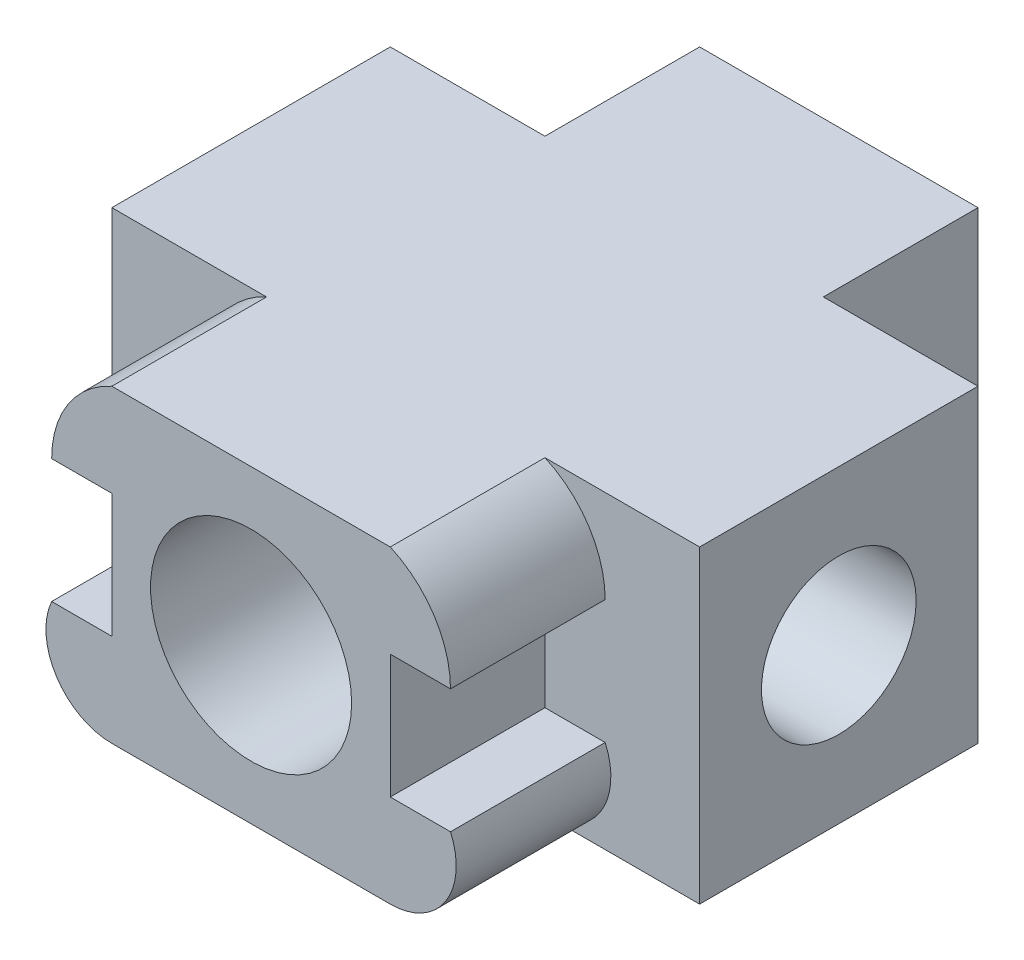
ISO-10303-21;
HEADER;
FILE_DESCRIPTION(('STEP AP214'),'2;1');
FILE_NAME('part.step','',(''),(''),'','','');
FILE_SCHEMA(('AUTOMOTIVE_DESIGN { 1 0 10303 214 1 1 1 1 }'));
ENDSEC;
DATA;
#1=APPLICATION_CONTEXT('core data for automotive mechanical design processes');
#2=APPLICATION_PROTOCOL_DEFINITION('international standard','automotive_design',2000,#1);
#3=PRODUCT_CONTEXT('',#1,'mechanical');
#4=PRODUCT('Part','Part','',(#3));
#5=PRODUCT_RELATED_PRODUCT_CATEGORY('part','',(#4));
#6=PRODUCT_DEFINITION_FORMATION('','',#4);
#7=PRODUCT_DEFINITION_CONTEXT('part definition',#1,'design');
#8=PRODUCT_DEFINITION('design','',#6,#7);
#9=PRODUCT_DEFINITION_SHAPE('','',#8);
#10=(LENGTH_UNIT() NAMED_UNIT(*) SI_UNIT(.MILLI.,.METRE.));
#11=(NAMED_UNIT(*) PLANE_ANGLE_UNIT() SI_UNIT($,.RADIAN.));
#12=(NAMED_UNIT(*) SI_UNIT($,.STERADIAN.) SOLID_ANGLE_UNIT());
#13=UNCERTAINTY_MEASURE_WITH_UNIT(LENGTH_MEASURE(1.E-05),#10,'distance_accuracy_value','');
#14=(GEOMETRIC_REPRESENTATION_CONTEXT(3) GLOBAL_UNCERTAINTY_ASSIGNED_CONTEXT((#13)) GLOBAL_UNIT_ASSIGNED_CONTEXT((#10,
#11,#12)) REPRESENTATION_CONTEXT('',''));
#15=CARTESIAN_POINT('',(0.,0.,0.));
#16=DIRECTION('',(0.,0.,1.));
#17=DIRECTION('',(1.,0.,0.));
#18=AXIS2_PLACEMENT_3D('',#15,#16,#17);
#19=CARTESIAN_POINT('',(20.,40.,36.));
#20=DIRECTION('',(0.,0.,-1.));
#21=DIRECTION('',(-1.,0.,0.));
#22=AXIS2_PLACEMENT_3D('',#19,#20,#21);
#23=PLANE('',#22);
#24=CARTESIAN_POINT('',(20.,8.52694245865046,36.));
#25=DIRECTION('',(0.,0.,1.));
#26=DIRECTION('',(1.,0.,0.));
#27=AXIS2_PLACEMENT_3D('',#24,#25,#26);
#28=CIRCLE('',#27,8.52694245865046);
#29=CARTESIAN_POINT('',(20.,0.,36.));
#30=VERTEX_POINT('',#29);
#31=CARTESIAN_POINT('',(12.2124060835447,12.,36.));
#32=VERTEX_POINT('',#31);
#33=EDGE_CURVE('E57',#30,#32,#28,.F.);
#34=ORIENTED_EDGE('',*,*,#33,.T.);
#35=DIRECTION('',(-1.,0.,0.));
#36=VECTOR('',#35,1.);
#37=CARTESIAN_POINT('',(0.,12.,36.));
#38=LINE('',#37,#36);
#39=CARTESIAN_POINT('',(20.,12.,36.));
#40=VERTEX_POINT('',#39);
#41=EDGE_CURVE('E64',#40,#32,#38,.T.);
#42=ORIENTED_EDGE('',*,*,#41,.F.);
#43=DIRECTION('',(0.,-1.,0.));
#44=VECTOR('',#43,1.);
#45=CARTESIAN_POINT('',(20.,40.,36.));
#46=LINE('',#45,#44);
#47=CARTESIAN_POINT('',(20.,28.,36.));
#48=VERTEX_POINT('',#47);
#49=EDGE_CURVE('E47',#48,#40,#46,.T.);
#50=ORIENTED_EDGE('',*,*,#49,.F.);
#51=DIRECTION('',(-1.,0.,0.));
#52=VECTOR('',#51,1.);
#53=CARTESIAN_POINT('',(0.,28.,36.));
#54=LINE('',#53,#52);
#55=CARTESIAN_POINT('',(12.2124060835447,28.,36.));
#56=VERTEX_POINT('',#55);
#57=EDGE_CURVE('E249',#48,#56,#54,.T.);
#58=ORIENTED_EDGE('',*,*,#57,.T.);
#59=CARTESIAN_POINT('',(25.3516774170943,28.,36.));
#60=DIRECTION('',(0.,0.,1.));
#61=DIRECTION('',(1.,0.,0.));
#62=AXIS2_PLACEMENT_3D('',#59,#60,#61);
#63=CIRCLE('',#62,13.1392713335496);
#64=CARTESIAN_POINT('',(20.,40.,36.));
#65=VERTEX_POINT('',#64);
#66=EDGE_CURVE('E248',#56,#65,#63,.F.);
#67=ORIENTED_EDGE('',*,*,#66,.T.);
#68=DIRECTION('',(1.,0.,0.));
#69=VECTOR('',#68,1.);
#70=CARTESIAN_POINT('',(20.,40.,36.));
#71=LINE('',#70,#69);
#72=CARTESIAN_POINT('',(0.,40.,36.));
#73=VERTEX_POINT('',#72);
#74=EDGE_CURVE('E262',#73,#65,#71,.T.);
#75=ORIENTED_EDGE('',*,*,#74,.F.);
#76=DIRECTION('',(0.,-1.,0.));
#77=VECTOR('',#76,1.);
#78=CARTESIAN_POINT('',(0.,40.,36.));
#79=LINE('',#78,#77);
#80=CARTESIAN_POINT('',(0.,0.,36.));
#81=VERTEX_POINT('',#80);
#82=EDGE_CURVE('E11',#73,#81,#79,.T.);
#83=ORIENTED_EDGE('',*,*,#82,.T.);
#84=DIRECTION('',(1.,0.,0.));
#85=VECTOR('',#84,1.);
#86=CARTESIAN_POINT('',(20.,0.,36.));
#87=LINE('',#86,#85);
#88=EDGE_CURVE('E192',#81,#30,#87,.T.);
#89=ORIENTED_EDGE('',*,*,#88,.T.);
#90=EDGE_LOOP('',(#34,#42,#50,#58,#67,#75,#83,#89));
#91=FACE_BOUND('',#90,.T.);
#92=ADVANCED_FACE('F41',(#91),#23,.F.);
#93=CARTESIAN_POINT('',(56.,40.,36.));
#94=DIRECTION('',(-1.,0.,0.));
#95=DIRECTION('',(0.,0.,1.));
#96=AXIS2_PLACEMENT_3D('',#93,#94,#95);
#97=PLANE('',#96);
#98=DIRECTION('',(0.,0.,1.));
#99=VECTOR('',#98,1.);
#100=CARTESIAN_POINT('',(56.,12.,36.));
#101=LINE('',#100,#99);
#102=CARTESIAN_POINT('',(56.,12.,36.));
#103=VERTEX_POINT('',#102);
#104=CARTESIAN_POINT('',(56.,12.,56.));
#105=VERTEX_POINT('',#104);
#106=EDGE_CURVE('E223',#103,#105,#101,.T.);
#107=ORIENTED_EDGE('',*,*,#106,.F.);
#108=DIRECTION('',(0.,-1.,0.));
#109=VECTOR('',#108,1.);
#110=CARTESIAN_POINT('',(56.,40.,36.));
#111=LINE('',#110,#109);
#112=CARTESIAN_POINT('',(56.,28.,36.));
#113=VERTEX_POINT('',#112);
#114=EDGE_CURVE('E328',#113,#103,#111,.T.);
#115=ORIENTED_EDGE('',*,*,#114,.F.);
#116=DIRECTION('',(0.,0.,1.));
#117=VECTOR('',#116,1.);
#118=CARTESIAN_POINT('',(56.,28.,36.));
#119=LINE('',#118,#117);
#120=CARTESIAN_POINT('',(56.,28.,56.));
#121=VERTEX_POINT('',#120);
#122=EDGE_CURVE('E244',#113,#121,#119,.T.);
#123=ORIENTED_EDGE('',*,*,#122,.T.);
#124=DIRECTION('',(0.,-1.,0.));
#125=VECTOR('',#124,1.);
#126=CARTESIAN_POINT('',(56.,40.,56.));
#127=LINE('',#126,#125);
#128=EDGE_CURVE('E335',#121,#105,#127,.T.);
#129=ORIENTED_EDGE('',*,*,#128,.T.);
#130=EDGE_LOOP('',(#107,#115,#123,#129));
#131=FACE_BOUND('',#130,.T.);
#132=ADVANCED_FACE('F404',(#131),#97,.F.);
#133=CARTESIAN_POINT('',(76.,40.,36.));
#134=DIRECTION('',(0.,0.,-1.));
#135=DIRECTION('',(-1.,0.,0.));
#136=AXIS2_PLACEMENT_3D('',#133,#134,#135);
#137=PLANE('',#136);
#138=DIRECTION('',(1.,0.,0.));
#139=VECTOR('',#138,1.);
#140=CARTESIAN_POINT('',(0.,12.,36.));
#141=LINE('',#140,#139);
#142=CARTESIAN_POINT('',(63.7875939164553,12.,36.));
#143=VERTEX_POINT('',#142);
#144=EDGE_CURVE('E217',#103,#143,#141,.T.);
#145=ORIENTED_EDGE('',*,*,#144,.T.);
#146=CARTESIAN_POINT('',(56.,8.52694245865045,36.));
#147=DIRECTION('',(0.,0.,1.));
#148=DIRECTION('',(1.,0.,0.));
#149=AXIS2_PLACEMENT_3D('',#146,#147,#148);
#150=CIRCLE('',#149,8.52694245865045);
#151=CARTESIAN_POINT('',(56.,0.,36.));
#152=VERTEX_POINT('',#151);
#153=EDGE_CURVE('E214',#152,#143,#150,.T.);
#154=ORIENTED_EDGE('',*,*,#153,.F.);
#155=DIRECTION('',(1.,0.,0.));
#156=VECTOR('',#155,1.);
#157=CARTESIAN_POINT('',(76.,0.,36.));
#158=LINE('',#157,#156);
#159=CARTESIAN_POINT('',(76.,0.,36.));
#160=VERTEX_POINT('',#159);
#161=EDGE_CURVE('E299',#152,#160,#158,.T.);
#162=ORIENTED_EDGE('',*,*,#161,.T.);
#163=DIRECTION('',(0.,-1.,0.));
#164=VECTOR('',#163,1.);
#165=CARTESIAN_POINT('',(76.,40.,36.));
#166=LINE('',#165,#164);
#167=CARTESIAN_POINT('',(76.,40.,36.));
#168=VERTEX_POINT('',#167);
#169=EDGE_CURVE('E326',#168,#160,#166,.T.);
#170=ORIENTED_EDGE('',*,*,#169,.F.);
#171=DIRECTION('',(1.,0.,0.));
#172=VECTOR('',#171,1.);
#173=CARTESIAN_POINT('',(76.,40.,36.));
#174=LINE('',#173,#172);
#175=CARTESIAN_POINT('',(56.,40.,36.));
#176=VERTEX_POINT('',#175);
#177=EDGE_CURVE('E280',#176,#168,#174,.T.);
#178=ORIENTED_EDGE('',*,*,#177,.F.);
#179=CARTESIAN_POINT('',(50.6483225829057,28.,36.));
#180=DIRECTION('',(0.,0.,1.));
#181=DIRECTION('',(1.,0.,0.));
#182=AXIS2_PLACEMENT_3D('',#179,#180,#181);
#183=CIRCLE('',#182,13.1392713335496);
#184=CARTESIAN_POINT('',(63.7875939164553,28.,36.));
#185=VERTEX_POINT('',#184);
#186=EDGE_CURVE('E231',#185,#176,#183,.T.);
#187=ORIENTED_EDGE('',*,*,#186,.F.);
#188=DIRECTION('',(1.,0.,0.));
#189=VECTOR('',#188,1.);
#190=CARTESIAN_POINT('',(0.,28.,36.));
#191=LINE('',#190,#189);
#192=EDGE_CURVE('E227',#113,#185,#191,.T.);
#193=ORIENTED_EDGE('',*,*,#192,.F.);
#194=ORIENTED_EDGE('',*,*,#114,.T.);
#195=EDGE_LOOP('',(#145,#154,#162,#170,#178,#187,#193,#194));
#196=FACE_BOUND('',#195,.T.);
#197=ADVANCED_FACE('F391',(#196),#137,.F.);
#198=CARTESIAN_POINT('',(20.,40.,56.));
#199=DIRECTION('',(1.,0.,0.));
#200=DIRECTION('',(0.,0.,-1.));
#201=AXIS2_PLACEMENT_3D('',#198,#199,#200);
#202=PLANE('',#201);
#203=ORIENTED_EDGE('',*,*,#49,.T.);
#204=DIRECTION('',(0.,0.,1.));
#205=VECTOR('',#204,1.);
#206=CARTESIAN_POINT('',(20.,12.,36.));
#207=LINE('',#206,#205);
#208=CARTESIAN_POINT('',(20.,12.,56.));
#209=VERTEX_POINT('',#208);
#210=EDGE_CURVE('E213',#40,#209,#207,.T.);
#211=ORIENTED_EDGE('',*,*,#210,.T.);
#212=DIRECTION('',(0.,-1.,0.));
#213=VECTOR('',#212,1.);
#214=CARTESIAN_POINT('',(20.,40.,56.));
#215=LINE('',#214,#213);
#216=CARTESIAN_POINT('',(20.,28.,56.));
#217=VERTEX_POINT('',#216);
#218=EDGE_CURVE('E331',#217,#209,#215,.T.);
#219=ORIENTED_EDGE('',*,*,#218,.F.);
#220=DIRECTION('',(0.,0.,1.));
#221=VECTOR('',#220,1.);
#222=CARTESIAN_POINT('',(20.,28.,36.));
#223=LINE('',#222,#221);
#224=EDGE_CURVE('E258',#48,#217,#223,.T.);
#225=ORIENTED_EDGE('',*,*,#224,.F.);
#226=EDGE_LOOP('',(#203,#211,#219,#225));
#227=FACE_BOUND('',#226,.T.);
#228=ADVANCED_FACE('F340',(#227),#202,.F.);
#229=CARTESIAN_POINT('',(0.,40.,36.));
#230=DIRECTION('',(1.,0.,0.));
#231=DIRECTION('',(0.,0.,-1.));
#232=AXIS2_PLACEMENT_3D('',#229,#230,#231);
#233=PLANE('',#232);
#234=CARTESIAN_POINT('',(0.,20.,18.));
#235=DIRECTION('',(1.,0.,0.));
#236=DIRECTION('',(0.,0.,-1.));
#237=AXIS2_PLACEMENT_3D('',#234,#235,#236);
#238=CIRCLE('',#237,10.);
#239=CARTESIAN_POINT('',(0.,20.,8.00000000000002));
#240=VERTEX_POINT('',#239);
#241=EDGE_CURVE('E344',#240,#240,#238,.T.);
#242=ORIENTED_EDGE('',*,*,#241,.T.);
#243=EDGE_LOOP('',(#242));
#244=FACE_BOUND('',#243,.T.);
#245=DIRECTION('',(0.,0.,1.));
#246=VECTOR('',#245,1.);
#247=CARTESIAN_POINT('',(0.,0.,36.));
#248=LINE('',#247,#246);
#249=CARTESIAN_POINT('',(0.,0.,0.));
#250=VERTEX_POINT('',#249);
#251=EDGE_CURVE('E256',#250,#81,#248,.T.);
#252=ORIENTED_EDGE('',*,*,#251,.T.);
#253=ORIENTED_EDGE('',*,*,#82,.F.);
#254=DIRECTION('',(0.,0.,1.));
#255=VECTOR('',#254,1.);
#256=CARTESIAN_POINT('',(0.,40.,36.));
#257=LINE('',#256,#255);
#258=CARTESIAN_POINT('',(0.,40.,0.));
#259=VERTEX_POINT('',#258);
#260=EDGE_CURVE('E261',#259,#73,#257,.T.);
#261=ORIENTED_EDGE('',*,*,#260,.F.);
#262=DIRECTION('',(0.,-1.,0.));
#263=VECTOR('',#262,1.);
#264=CARTESIAN_POINT('',(0.,40.,0.));
#265=LINE('',#264,#263);
#266=EDGE_CURVE('E292',#259,#250,#265,.T.);
#267=ORIENTED_EDGE('',*,*,#266,.T.);
#268=EDGE_LOOP('',(#252,#253,#261,#267));
#269=FACE_BOUND('',#268,.T.);
#270=ADVANCED_FACE('F43',(#244,#269),#233,.F.);
#271=CARTESIAN_POINT('',(56.,40.,56.));
#272=DIRECTION('',(0.,0.,-1.));
#273=DIRECTION('',(-1.,0.,0.));
#274=AXIS2_PLACEMENT_3D('',#271,#272,#273);
#275=PLANE('',#274);
#276=CARTESIAN_POINT('',(38.,20.,56.));
#277=DIRECTION('',(0.,0.,1.));
#278=DIRECTION('',(1.,0.,0.));
#279=AXIS2_PLACEMENT_3D('',#276,#277,#278);
#280=CIRCLE('',#279,13.);
#281=CARTESIAN_POINT('',(51.,20.,56.));
#282=VERTEX_POINT('',#281);
#283=EDGE_CURVE('E202',#282,#282,#280,.T.);
#284=ORIENTED_EDGE('',*,*,#283,.F.);
#285=EDGE_LOOP('',(#284));
#286=FACE_BOUND('',#285,.T.);
#287=DIRECTION('',(1.,0.,0.));
#288=VECTOR('',#287,1.);
#289=CARTESIAN_POINT('',(56.,0.,56.));
#290=LINE('',#289,#288);
#291=CARTESIAN_POINT('',(20.,0.,56.));
#292=VERTEX_POINT('',#291);
#293=CARTESIAN_POINT('',(56.,0.,56.));
#294=VERTEX_POINT('',#293);
#295=EDGE_CURVE('E176',#292,#294,#290,.T.);
#296=ORIENTED_EDGE('',*,*,#295,.T.);
#297=CARTESIAN_POINT('',(56.,8.52694245865045,56.));
#298=DIRECTION('',(0.,0.,1.));
#299=DIRECTION('',(1.,0.,0.));
#300=AXIS2_PLACEMENT_3D('',#297,#298,#299);
#301=CIRCLE('',#300,8.52694245865045);
#302=CARTESIAN_POINT('',(63.7875939164553,12.,56.));
#303=VERTEX_POINT('',#302);
#304=EDGE_CURVE('E215',#294,#303,#301,.T.);
#305=ORIENTED_EDGE('',*,*,#304,.T.);
#306=DIRECTION('',(1.,0.,0.));
#307=VECTOR('',#306,1.);
#308=CARTESIAN_POINT('',(0.,12.,56.));
#309=LINE('',#308,#307);
#310=EDGE_CURVE('E218',#105,#303,#309,.T.);
#311=ORIENTED_EDGE('',*,*,#310,.F.);
#312=ORIENTED_EDGE('',*,*,#128,.F.);
#313=DIRECTION('',(1.,0.,0.));
#314=VECTOR('',#313,1.);
#315=CARTESIAN_POINT('',(0.,28.,56.));
#316=LINE('',#315,#314);
#317=CARTESIAN_POINT('',(63.7875939164553,28.,56.));
#318=VERTEX_POINT('',#317);
#319=EDGE_CURVE('E230',#121,#318,#316,.T.);
#320=ORIENTED_EDGE('',*,*,#319,.T.);
#321=CARTESIAN_POINT('',(50.6483225829057,28.,56.));
#322=DIRECTION('',(0.,0.,1.));
#323=DIRECTION('',(1.,0.,0.));
#324=AXIS2_PLACEMENT_3D('',#321,#322,#323);
#325=CIRCLE('',#324,13.1392713335496);
#326=CARTESIAN_POINT('',(56.,40.,56.));
#327=VERTEX_POINT('',#326);
#328=EDGE_CURVE('E234',#318,#327,#325,.T.);
#329=ORIENTED_EDGE('',*,*,#328,.T.);
#330=DIRECTION('',(1.,0.,0.));
#331=VECTOR('',#330,1.);
#332=CARTESIAN_POINT('',(56.,40.,56.));
#333=LINE('',#332,#331);
#334=CARTESIAN_POINT('',(20.,40.,56.));
#335=VERTEX_POINT('',#334);
#336=EDGE_CURVE('E271',#335,#327,#333,.T.);
#337=ORIENTED_EDGE('',*,*,#336,.F.);
#338=CARTESIAN_POINT('',(25.3516774170943,28.,56.));
#339=DIRECTION('',(0.,0.,1.));
#340=DIRECTION('',(1.,0.,0.));
#341=AXIS2_PLACEMENT_3D('',#338,#339,#340);
#342=CIRCLE('',#341,13.1392713335496);
#343=CARTESIAN_POINT('',(12.2124060835447,28.,56.));
#344=VERTEX_POINT('',#343);
#345=EDGE_CURVE('E243',#344,#335,#342,.F.);
#346=ORIENTED_EDGE('',*,*,#345,.F.);
#347=DIRECTION('',(-1.,0.,0.));
#348=VECTOR('',#347,1.);
#349=CARTESIAN_POINT('',(0.,28.,56.));
#350=LINE('',#349,#348);
#351=EDGE_CURVE('E247',#217,#344,#350,.T.);
#352=ORIENTED_EDGE('',*,*,#351,.F.);
#353=ORIENTED_EDGE('',*,*,#218,.T.);
#354=DIRECTION('',(-1.,0.,0.));
#355=VECTOR('',#354,1.);
#356=CARTESIAN_POINT('',(0.,12.,56.));
#357=LINE('',#356,#355);
#358=CARTESIAN_POINT('',(12.2124060835447,12.,56.));
#359=VERTEX_POINT('',#358);
#360=EDGE_CURVE('E199',#209,#359,#357,.T.);
#361=ORIENTED_EDGE('',*,*,#360,.T.);
#362=CARTESIAN_POINT('',(20.,8.52694245865046,56.));
#363=DIRECTION('',(0.,0.,1.));
#364=DIRECTION('',(1.,0.,0.));
#365=AXIS2_PLACEMENT_3D('',#362,#363,#364);
#366=CIRCLE('',#365,8.52694245865046);
#367=EDGE_CURVE('E191',#292,#359,#366,.F.);
#368=ORIENTED_EDGE('',*,*,#367,.F.);
#369=EDGE_LOOP('',(#296,#305,#311,#312,#320,#329,#337,#346,#352,#353,#361,#368));
#370=FACE_BOUND('',#369,.T.);
#371=ADVANCED_FACE('F197',(#286,#370),#275,.F.);
#372=CARTESIAN_POINT('',(76.,40.,0.));
#373=DIRECTION('',(-1.,0.,0.));
#374=DIRECTION('',(0.,0.,1.));
#375=AXIS2_PLACEMENT_3D('',#372,#373,#374);
#376=PLANE('',#375);
#377=CARTESIAN_POINT('',(76.,20.,18.));
#378=DIRECTION('',(1.,0.,0.));
#379=DIRECTION('',(0.,0.,-1.));
#380=AXIS2_PLACEMENT_3D('',#377,#378,#379);
#381=CIRCLE('',#380,10.);
#382=CARTESIAN_POINT('',(76.,20.,7.99999999999999));
#383=VERTEX_POINT('',#382);
#384=EDGE_CURVE('E347',#383,#383,#381,.T.);
#385=ORIENTED_EDGE('',*,*,#384,.F.);
#386=EDGE_LOOP('',(#385));
#387=FACE_BOUND('',#386,.T.);
#388=DIRECTION('',(0.,0.,-1.));
#389=VECTOR('',#388,1.);
#390=CARTESIAN_POINT('',(76.,0.,0.));
#391=LINE('',#390,#389);
#392=CARTESIAN_POINT('',(76.,0.,0.));
#393=VERTEX_POINT('',#392);
#394=EDGE_CURVE('E300',#160,#393,#391,.T.);
#395=ORIENTED_EDGE('',*,*,#394,.T.);
#396=DIRECTION('',(0.,-1.,0.));
#397=VECTOR('',#396,1.);
#398=CARTESIAN_POINT('',(76.,40.,0.));
#399=LINE('',#398,#397);
#400=CARTESIAN_POINT('',(76.,40.,0.));
#401=VERTEX_POINT('',#400);
#402=EDGE_CURVE('E323',#401,#393,#399,.T.);
#403=ORIENTED_EDGE('',*,*,#402,.F.);
#404=DIRECTION('',(0.,0.,-1.));
#405=VECTOR('',#404,1.);
#406=CARTESIAN_POINT('',(76.,40.,0.));
#407=LINE('',#406,#405);
#408=EDGE_CURVE('E276',#168,#401,#407,.T.);
#409=ORIENTED_EDGE('',*,*,#408,.F.);
#410=ORIENTED_EDGE('',*,*,#169,.T.);
#411=EDGE_LOOP('',(#395,#403,#409,#410));
#412=FACE_BOUND('',#411,.T.);
#413=ADVANCED_FACE('F363',(#387,#412),#376,.F.);
#414=CARTESIAN_POINT('',(56.,40.,0.));
#415=DIRECTION('',(0.,0.,1.));
#416=DIRECTION('',(1.,0.,0.));
#417=AXIS2_PLACEMENT_3D('',#414,#415,#416);
#418=PLANE('',#417);
#419=DIRECTION('',(-1.,0.,0.));
#420=VECTOR('',#419,1.);
#421=CARTESIAN_POINT('',(56.,0.,0.));
#422=LINE('',#421,#420);
#423=CARTESIAN_POINT('',(56.,0.,0.));
#424=VERTEX_POINT('',#423);
#425=EDGE_CURVE('E297',#393,#424,#422,.T.);
#426=ORIENTED_EDGE('',*,*,#425,.T.);
#427=DIRECTION('',(0.,-1.,0.));
#428=VECTOR('',#427,1.);
#429=CARTESIAN_POINT('',(56.,40.,0.));
#430=LINE('',#429,#428);
#431=CARTESIAN_POINT('',(56.,40.,0.));
#432=VERTEX_POINT('',#431);
#433=EDGE_CURVE('E319',#432,#424,#430,.T.);
#434=ORIENTED_EDGE('',*,*,#433,.F.);
#435=DIRECTION('',(-1.,0.,0.));
#436=VECTOR('',#435,1.);
#437=CARTESIAN_POINT('',(56.,40.,0.));
#438=LINE('',#437,#436);
#439=EDGE_CURVE('E284',#401,#432,#438,.T.);
#440=ORIENTED_EDGE('',*,*,#439,.F.);
#441=ORIENTED_EDGE('',*,*,#402,.T.);
#442=EDGE_LOOP('',(#426,#434,#440,#441));
#443=FACE_BOUND('',#442,.T.);
#444=ADVANCED_FACE('F365',(#443),#418,.F.);
#445=CARTESIAN_POINT('',(56.,40.,-20.));
#446=DIRECTION('',(-1.,0.,0.));
#447=DIRECTION('',(0.,0.,1.));
#448=AXIS2_PLACEMENT_3D('',#445,#446,#447);
#449=PLANE('',#448);
#450=DIRECTION('',(0.,0.,-1.));
#451=VECTOR('',#450,1.);
#452=CARTESIAN_POINT('',(56.,0.,-20.));
#453=LINE('',#452,#451);
#454=CARTESIAN_POINT('',(56.,0.,-20.));
#455=VERTEX_POINT('',#454);
#456=EDGE_CURVE('E305',#424,#455,#453,.T.);
#457=ORIENTED_EDGE('',*,*,#456,.T.);
#458=DIRECTION('',(0.,-1.,0.));
#459=VECTOR('',#458,1.);
#460=CARTESIAN_POINT('',(56.,40.,-20.));
#461=LINE('',#460,#459);
#462=CARTESIAN_POINT('',(56.,40.,-20.));
#463=VERTEX_POINT('',#462);
#464=EDGE_CURVE('E320',#463,#455,#461,.T.);
#465=ORIENTED_EDGE('',*,*,#464,.F.);
#466=DIRECTION('',(0.,0.,-1.));
#467=VECTOR('',#466,1.);
#468=CARTESIAN_POINT('',(56.,40.,-20.));
#469=LINE('',#468,#467);
#470=EDGE_CURVE('E285',#432,#463,#469,.T.);
#471=ORIENTED_EDGE('',*,*,#470,.F.);
#472=ORIENTED_EDGE('',*,*,#433,.T.);
#473=EDGE_LOOP('',(#457,#465,#471,#472));
#474=FACE_BOUND('',#473,.T.);
#475=ADVANCED_FACE('F377',(#474),#449,.F.);
#476=CARTESIAN_POINT('',(20.,40.,-20.));
#477=DIRECTION('',(0.,0.,1.));
#478=DIRECTION('',(1.,0.,0.));
#479=AXIS2_PLACEMENT_3D('',#476,#477,#478);
#480=PLANE('',#479);
#481=DIRECTION('',(-1.,0.,0.));
#482=VECTOR('',#481,1.);
#483=CARTESIAN_POINT('',(20.,0.,-20.));
#484=LINE('',#483,#482);
#485=CARTESIAN_POINT('',(20.,0.,-20.));
#486=VERTEX_POINT('',#485);
#487=EDGE_CURVE('E304',#455,#486,#484,.T.);
#488=ORIENTED_EDGE('',*,*,#487,.T.);
#489=DIRECTION('',(0.,-1.,0.));
#490=VECTOR('',#489,1.);
#491=CARTESIAN_POINT('',(20.,40.,-20.));
#492=LINE('',#491,#490);
#493=CARTESIAN_POINT('',(20.,40.,-20.));
#494=VERTEX_POINT('',#493);
#495=EDGE_CURVE('E314',#494,#486,#492,.T.);
#496=ORIENTED_EDGE('',*,*,#495,.F.);
#497=DIRECTION('',(-1.,0.,0.));
#498=VECTOR('',#497,1.);
#499=CARTESIAN_POINT('',(20.,40.,-20.));
#500=LINE('',#499,#498);
#501=EDGE_CURVE('E282',#463,#494,#500,.T.);
#502=ORIENTED_EDGE('',*,*,#501,.F.);
#503=ORIENTED_EDGE('',*,*,#464,.T.);
#504=EDGE_LOOP('',(#488,#496,#502,#503));
#505=FACE_BOUND('',#504,.T.);
#506=ADVANCED_FACE('F382',(#505),#480,.F.);
#507=CARTESIAN_POINT('',(20.,40.,0.));
#508=DIRECTION('',(1.,0.,0.));
#509=DIRECTION('',(0.,0.,-1.));
#510=AXIS2_PLACEMENT_3D('',#507,#508,#509);
#511=PLANE('',#510);
#512=DIRECTION('',(0.,0.,1.));
#513=VECTOR('',#512,1.);
#514=CARTESIAN_POINT('',(20.,0.,0.));
#515=LINE('',#514,#513);
#516=CARTESIAN_POINT('',(20.,0.,0.));
#517=VERTEX_POINT('',#516);
#518=EDGE_CURVE('E308',#486,#517,#515,.T.);
#519=ORIENTED_EDGE('',*,*,#518,.T.);
#520=DIRECTION('',(0.,-1.,0.));
#521=VECTOR('',#520,1.);
#522=CARTESIAN_POINT('',(20.,40.,0.));
#523=LINE('',#522,#521);
#524=CARTESIAN_POINT('',(20.,40.,0.));
#525=VERTEX_POINT('',#524);
#526=EDGE_CURVE('E313',#525,#517,#523,.T.);
#527=ORIENTED_EDGE('',*,*,#526,.F.);
#528=DIRECTION('',(0.,0.,1.));
#529=VECTOR('',#528,1.);
#530=CARTESIAN_POINT('',(20.,40.,0.));
#531=LINE('',#530,#529);
#532=EDGE_CURVE('E290',#494,#525,#531,.T.);
#533=ORIENTED_EDGE('',*,*,#532,.F.);
#534=ORIENTED_EDGE('',*,*,#495,.T.);
#535=EDGE_LOOP('',(#519,#527,#533,#534));
#536=FACE_BOUND('',#535,.T.);
#537=ADVANCED_FACE('F446',(#536),#511,.F.);
#538=CARTESIAN_POINT('',(0.,40.,0.));
#539=DIRECTION('',(0.,0.,1.));
#540=DIRECTION('',(1.,0.,0.));
#541=AXIS2_PLACEMENT_3D('',#538,#539,#540);
#542=PLANE('',#541);
#543=DIRECTION('',(-1.,0.,0.));
#544=VECTOR('',#543,1.);
#545=CARTESIAN_POINT('',(0.,0.,0.));
#546=LINE('',#545,#544);
#547=EDGE_CURVE('E264',#517,#250,#546,.T.);
#548=ORIENTED_EDGE('',*,*,#547,.T.);
#549=ORIENTED_EDGE('',*,*,#266,.F.);
#550=DIRECTION('',(-1.,0.,0.));
#551=VECTOR('',#550,1.);
#552=CARTESIAN_POINT('',(0.,40.,0.));
#553=LINE('',#552,#551);
#554=EDGE_CURVE('E289',#525,#259,#553,.T.);
#555=ORIENTED_EDGE('',*,*,#554,.F.);
#556=ORIENTED_EDGE('',*,*,#526,.T.);
#557=EDGE_LOOP('',(#548,#549,#555,#556));
#558=FACE_BOUND('',#557,.T.);
#559=ADVANCED_FACE('F447',(#558),#542,.F.);
#560=CARTESIAN_POINT('',(0.,40.,0.));
#561=DIRECTION('',(0.,-1.,0.));
#562=DIRECTION('',(0.,0.,-1.));
#563=AXIS2_PLACEMENT_3D('',#560,#561,#562);
#564=PLANE('',#563);
#565=ORIENTED_EDGE('',*,*,#260,.T.);
#566=ORIENTED_EDGE('',*,*,#74,.T.);
#567=DIRECTION('',(0.,0.,1.));
#568=VECTOR('',#567,1.);
#569=CARTESIAN_POINT('',(20.,40.,56.));
#570=LINE('',#569,#568);
#571=EDGE_CURVE('E268',#65,#335,#570,.T.);
#572=ORIENTED_EDGE('',*,*,#571,.T.);
#573=ORIENTED_EDGE('',*,*,#336,.T.);
#574=DIRECTION('',(0.,0.,-1.));
#575=VECTOR('',#574,1.);
#576=CARTESIAN_POINT('',(56.,40.,36.));
#577=LINE('',#576,#575);
#578=EDGE_CURVE('E273',#327,#176,#577,.T.);
#579=ORIENTED_EDGE('',*,*,#578,.T.);
#580=ORIENTED_EDGE('',*,*,#177,.T.);
#581=ORIENTED_EDGE('',*,*,#408,.T.);
#582=ORIENTED_EDGE('',*,*,#439,.T.);
#583=ORIENTED_EDGE('',*,*,#470,.T.);
#584=ORIENTED_EDGE('',*,*,#501,.T.);
#585=ORIENTED_EDGE('',*,*,#532,.T.);
#586=ORIENTED_EDGE('',*,*,#554,.T.);
#587=EDGE_LOOP('',(#565,#566,#572,#573,#579,#580,#581,#582,#583,#584,#585,#586));
#588=FACE_BOUND('',#587,.T.);
#589=ADVANCED_FACE('F390',(#588),#564,.F.);
#590=CARTESIAN_POINT('',(0.,0.,0.));
#591=DIRECTION('',(0.,-1.,0.));
#592=DIRECTION('',(0.,0.,-1.));
#593=AXIS2_PLACEMENT_3D('',#590,#591,#592);
#594=PLANE('',#593);
#595=ORIENTED_EDGE('',*,*,#251,.F.);
#596=ORIENTED_EDGE('',*,*,#547,.F.);
#597=ORIENTED_EDGE('',*,*,#518,.F.);
#598=ORIENTED_EDGE('',*,*,#487,.F.);
#599=ORIENTED_EDGE('',*,*,#456,.F.);
#600=ORIENTED_EDGE('',*,*,#425,.F.);
#601=ORIENTED_EDGE('',*,*,#394,.F.);
#602=ORIENTED_EDGE('',*,*,#161,.F.);
#603=DIRECTION('',(0.,0.,-1.));
#604=VECTOR('',#603,1.);
#605=CARTESIAN_POINT('',(56.,0.,36.));
#606=LINE('',#605,#604);
#607=EDGE_CURVE('E184',#294,#152,#606,.T.);
#608=ORIENTED_EDGE('',*,*,#607,.F.);
#609=ORIENTED_EDGE('',*,*,#295,.F.);
#610=DIRECTION('',(0.,0.,1.));
#611=VECTOR('',#610,1.);
#612=CARTESIAN_POINT('',(20.,0.,56.));
#613=LINE('',#612,#611);
#614=EDGE_CURVE('E185',#30,#292,#613,.T.);
#615=ORIENTED_EDGE('',*,*,#614,.F.);
#616=ORIENTED_EDGE('',*,*,#88,.F.);
#617=EDGE_LOOP('',(#595,#596,#597,#598,#599,#600,#601,#602,#608,#609,#615,#616));
#618=FACE_BOUND('',#617,.T.);
#619=ADVANCED_FACE('F182',(#618),#594,.T.);
#620=CARTESIAN_POINT('',(25.3516774170943,28.,36.));
#621=DIRECTION('',(0.,0.,1.));
#622=DIRECTION('',(1.,0.,0.));
#623=AXIS2_PLACEMENT_3D('',#620,#621,#622);
#624=CYLINDRICAL_SURFACE('',#623,13.1392713335496);
#625=ORIENTED_EDGE('',*,*,#345,.T.);
#626=ORIENTED_EDGE('',*,*,#571,.F.);
#627=ORIENTED_EDGE('',*,*,#66,.F.);
#628=DIRECTION('',(0.,0.,1.));
#629=VECTOR('',#628,1.);
#630=CARTESIAN_POINT('',(12.2124060835447,28.,36.));
#631=LINE('',#630,#629);
#632=EDGE_CURVE('E251',#56,#344,#631,.T.);
#633=ORIENTED_EDGE('',*,*,#632,.T.);
#634=EDGE_LOOP('',(#625,#626,#627,#633));
#635=FACE_BOUND('',#634,.T.);
#636=ADVANCED_FACE('F414',(#635),#624,.T.);
#637=CARTESIAN_POINT('',(0.,28.,36.));
#638=DIRECTION('',(0.,1.,0.));
#639=DIRECTION('',(0.,0.,1.));
#640=AXIS2_PLACEMENT_3D('',#637,#638,#639);
#641=PLANE('',#640);
#642=ORIENTED_EDGE('',*,*,#351,.T.);
#643=ORIENTED_EDGE('',*,*,#632,.F.);
#644=ORIENTED_EDGE('',*,*,#57,.F.);
#645=ORIENTED_EDGE('',*,*,#224,.T.);
#646=EDGE_LOOP('',(#642,#643,#644,#645));
#647=FACE_BOUND('',#646,.T.);
#648=ADVANCED_FACE('F418',(#647),#641,.F.);
#649=CARTESIAN_POINT('',(0.,28.,36.));
#650=DIRECTION('',(0.,-1.,0.));
#651=DIRECTION('',(1.,0.,0.));
#652=AXIS2_PLACEMENT_3D('',#649,#650,#651);
#653=PLANE('',#652);
#654=ORIENTED_EDGE('',*,*,#319,.F.);
#655=ORIENTED_EDGE('',*,*,#122,.F.);
#656=ORIENTED_EDGE('',*,*,#192,.T.);
#657=DIRECTION('',(0.,0.,1.));
#658=VECTOR('',#657,1.);
#659=CARTESIAN_POINT('',(63.7875939164553,28.,36.));
#660=LINE('',#659,#658);
#661=EDGE_CURVE('E237',#185,#318,#660,.T.);
#662=ORIENTED_EDGE('',*,*,#661,.T.);
#663=EDGE_LOOP('',(#654,#655,#656,#662));
#664=FACE_BOUND('',#663,.T.);
#665=ADVANCED_FACE('F406',(#664),#653,.T.);
#666=CARTESIAN_POINT('',(50.6483225829057,28.,36.));
#667=DIRECTION('',(0.,0.,1.));
#668=DIRECTION('',(1.,0.,0.));
#669=AXIS2_PLACEMENT_3D('',#666,#667,#668);
#670=CYLINDRICAL_SURFACE('',#669,13.1392713335496);
#671=ORIENTED_EDGE('',*,*,#328,.F.);
#672=ORIENTED_EDGE('',*,*,#661,.F.);
#673=ORIENTED_EDGE('',*,*,#186,.T.);
#674=ORIENTED_EDGE('',*,*,#578,.F.);
#675=EDGE_LOOP('',(#671,#672,#673,#674));
#676=FACE_BOUND('',#675,.T.);
#677=ADVANCED_FACE('F424',(#676),#670,.T.);
#678=CARTESIAN_POINT('',(0.,12.,36.));
#679=DIRECTION('',(0.,-1.,0.));
#680=DIRECTION('',(1.,0.,0.));
#681=AXIS2_PLACEMENT_3D('',#678,#679,#680);
#682=PLANE('',#681);
#683=ORIENTED_EDGE('',*,*,#310,.T.);
#684=DIRECTION('',(0.,0.,1.));
#685=VECTOR('',#684,1.);
#686=CARTESIAN_POINT('',(63.7875939164553,12.,36.));
#687=LINE('',#686,#685);
#688=EDGE_CURVE('E222',#143,#303,#687,.T.);
#689=ORIENTED_EDGE('',*,*,#688,.F.);
#690=ORIENTED_EDGE('',*,*,#144,.F.);
#691=ORIENTED_EDGE('',*,*,#106,.T.);
#692=EDGE_LOOP('',(#683,#689,#690,#691));
#693=FACE_BOUND('',#692,.T.);
#694=ADVANCED_FACE('F402',(#693),#682,.F.);
#695=CARTESIAN_POINT('',(56.,8.52694245865045,36.));
#696=DIRECTION('',(0.,0.,1.));
#697=DIRECTION('',(1.,0.,0.));
#698=AXIS2_PLACEMENT_3D('',#695,#696,#697);
#699=CYLINDRICAL_SURFACE('',#698,8.52694245865045);
#700=ORIENTED_EDGE('',*,*,#304,.F.);
#701=ORIENTED_EDGE('',*,*,#607,.T.);
#702=ORIENTED_EDGE('',*,*,#153,.T.);
#703=ORIENTED_EDGE('',*,*,#688,.T.);
#704=EDGE_LOOP('',(#700,#701,#702,#703));
#705=FACE_BOUND('',#704,.T.);
#706=ADVANCED_FACE('F400',(#705),#699,.T.);
#707=CARTESIAN_POINT('',(20.,8.52694245865046,36.));
#708=DIRECTION('',(0.,0.,1.));
#709=DIRECTION('',(1.,0.,0.));
#710=AXIS2_PLACEMENT_3D('',#707,#708,#709);
#711=CYLINDRICAL_SURFACE('',#710,8.52694245865046);
#712=ORIENTED_EDGE('',*,*,#367,.T.);
#713=DIRECTION('',(0.,0.,1.));
#714=VECTOR('',#713,1.);
#715=CARTESIAN_POINT('',(12.2124060835447,12.,36.));
#716=LINE('',#715,#714);
#717=EDGE_CURVE('E209',#32,#359,#716,.T.);
#718=ORIENTED_EDGE('',*,*,#717,.F.);
#719=ORIENTED_EDGE('',*,*,#33,.F.);
#720=ORIENTED_EDGE('',*,*,#614,.T.);
#721=EDGE_LOOP('',(#712,#718,#719,#720));
#722=FACE_BOUND('',#721,.T.);
#723=ADVANCED_FACE('F195',(#722),#711,.T.);
#724=CARTESIAN_POINT('',(0.,12.,36.));
#725=DIRECTION('',(0.,1.,0.));
#726=DIRECTION('',(-1.,0.,0.));
#727=AXIS2_PLACEMENT_3D('',#724,#725,#726);
#728=PLANE('',#727);
#729=ORIENTED_EDGE('',*,*,#360,.F.);
#730=ORIENTED_EDGE('',*,*,#210,.F.);
#731=ORIENTED_EDGE('',*,*,#41,.T.);
#732=ORIENTED_EDGE('',*,*,#717,.T.);
#733=EDGE_LOOP('',(#729,#730,#731,#732));
#734=FACE_BOUND('',#733,.T.);
#735=ADVANCED_FACE('F343',(#734),#728,.T.);
#736=CARTESIAN_POINT('',(38.,20.,36.));
#737=DIRECTION('',(0.,0.,1.));
#738=DIRECTION('',(1.,0.,0.));
#739=AXIS2_PLACEMENT_3D('',#736,#737,#738);
#740=CYLINDRICAL_SURFACE('',#739,13.);
#741=CARTESIAN_POINT('',(38.,20.,36.));
#742=DIRECTION('',(0.,0.,1.));
#743=DIRECTION('',(1.,0.,0.));
#744=AXIS2_PLACEMENT_3D('',#741,#742,#743);
#745=CIRCLE('',#744,13.);
#746=CARTESIAN_POINT('',(51.,20.,36.));
#747=VERTEX_POINT('',#746);
#748=EDGE_CURVE('E203',#747,#747,#745,.T.);
#749=ORIENTED_EDGE('',*,*,#748,.F.);
#750=EDGE_LOOP('',(#749));
#751=FACE_BOUND('',#750,.T.);
#752=ORIENTED_EDGE('',*,*,#283,.T.);
#753=EDGE_LOOP('',(#752));
#754=FACE_BOUND('',#753,.T.);
#755=ADVANCED_FACE('F529',(#751,#754),#740,.F.);
#756=CARTESIAN_POINT('',(38.,20.,36.));
#757=DIRECTION('',(0.,0.,1.));
#758=DIRECTION('',(1.,0.,0.));
#759=AXIS2_PLACEMENT_3D('',#756,#757,#758);
#760=PLANE('',#759);
#761=ORIENTED_EDGE('',*,*,#748,.T.);
#762=EDGE_LOOP('',(#761));
#763=FACE_BOUND('',#762,.T.);
#764=ADVANCED_FACE('F360',(#763),#760,.T.);
#765=CARTESIAN_POINT('',(0.,20.,18.));
#766=DIRECTION('',(1.,0.,0.));
#767=DIRECTION('',(0.,0.,-1.));
#768=AXIS2_PLACEMENT_3D('',#765,#766,#767);
#769=CYLINDRICAL_SURFACE('',#768,10.);
#770=ORIENTED_EDGE('',*,*,#241,.F.);
#771=EDGE_LOOP('',(#770));
#772=FACE_BOUND('',#771,.T.);
#773=ORIENTED_EDGE('',*,*,#384,.T.);
#774=EDGE_LOOP('',(#773));
#775=FACE_BOUND('',#774,.T.);
#776=ADVANCED_FACE('F353',(#772,#775),#769,.F.);
#777=CLOSED_SHELL('',(#92,#132,#197,#228,#270,#371,#413,#444,#475,#506,#537,#559,#589,#619,#636,
#648,#665,#677,#694,#706,#723,#735,#755,#764,#776));
#778=MANIFOLD_SOLID_BREP('B2',#777);
#779=ADVANCED_BREP_SHAPE_REPRESENTATION('',(#18,#778),#14);
#780=SHAPE_DEFINITION_REPRESENTATION(#9,#779);
ENDSEC;
END-ISO-10303-21;
